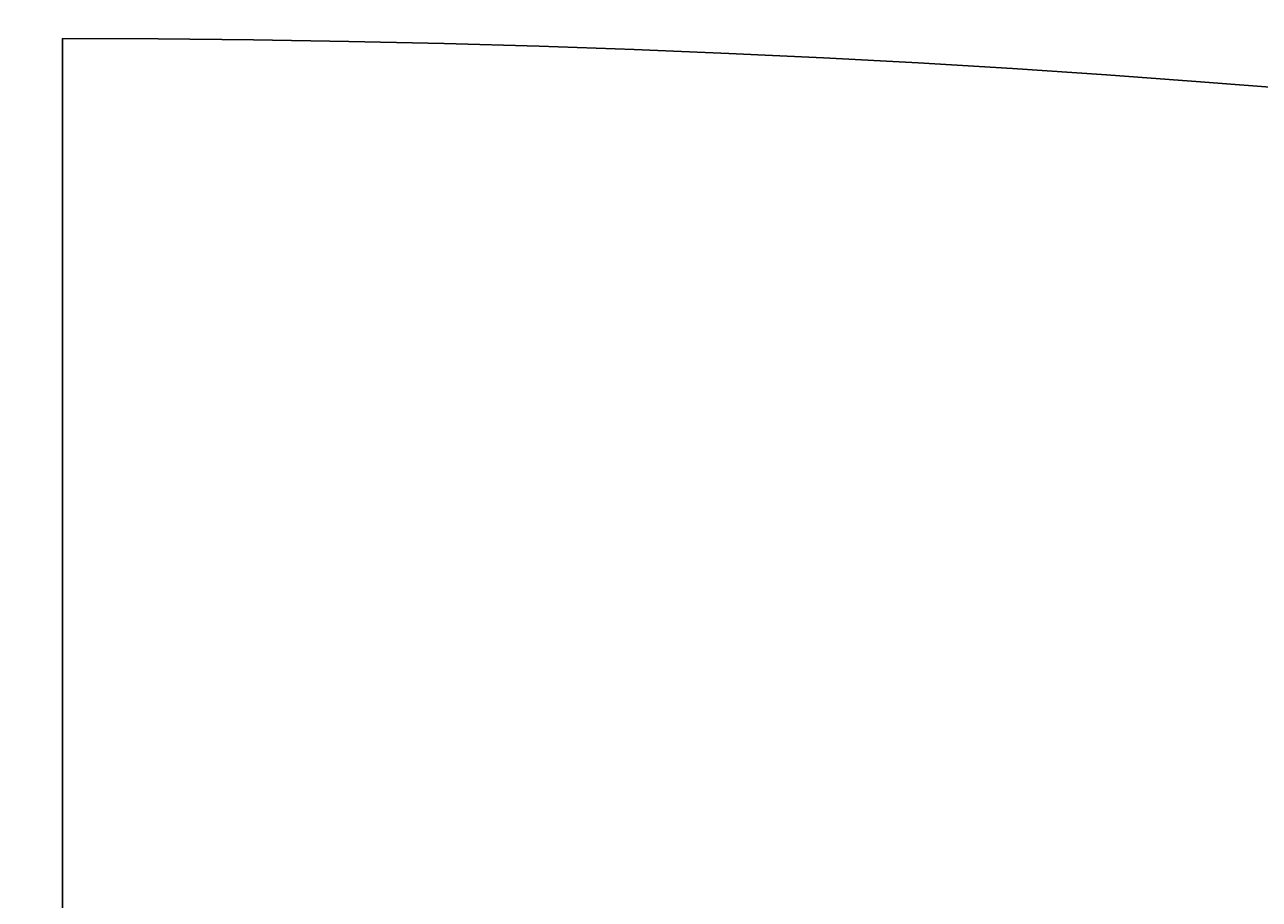
# Model space of a CAD drawing. Units: millimetres. Extents: x 19292 to 100733, y 12374 to 26974.
# Tile 8 of 24: x 29467 to 29528, y 15599 to 15642. Entities that reach past the tile are written whole.
import ezdxf

# ---------------------------------------------------------------- set-up
doc = ezdxf.new("R2010")
doc.units = ezdxf.units.MM
doc.layers.add('A-ANNO-DIMS', color=2, linetype='Continuous', lineweight=18)
doc.layers.add('A-DOOR', color=4, linetype='Continuous', lineweight=25)
doc.styles.get("Standard").update_dxf_attribs({"font": 'arial.ttf'})
doc.dimstyles.get("Standard").update_dxf_attribs({"dimtxt": 0.18, "dimasz": 0.18, "dimexe": 0.18, "dimexo": 0.0625, "dimgap": 0.09, "dimtad": 0, "dimtih": 1, "dimtoh": 1, "dimdec": 4, "dimzin": 0, "dimdsep": 46, "dimtxsty": 'Standard', "dimcen": 0.09, "dimadec": 0, "dimazin": 0, "dimtfac": 1, "dimtdec": 4, "dimtofl": 0, "dimtmove": 0, "dimatfit": 3, "dimfxl": 1, "dimtolj": 1, "dimtzin": 0, "dimarcsym": 0})

# ---------------------------------------------------------------- blocks, each defined once
blk = doc.blocks.new('*D79')
at = {"layer": 'A-ANNO-DIMS', "color": 0, "lineweight": -2, "transparency": 16777216}
for p, q in [((22694.132, 22860.662), (22694.132, 12808.813)), ((36144.169, 15985.662), (36144.169, 12808.813)), ((22694.312, 12808.993), (29418.731, 12808.993)), ((36143.989, 12808.993), (29419.571, 12808.993))]:
    blk.add_line(p, q, dxfattribs=at)
at = {"layer": 'A-ANNO-DIMS', "color": 0, "transparency": 16777216}
for points in [[(22694.312, 12809.023), (22694.312, 12808.963), (22694.132, 12808.993)], [(36143.989, 12809.023), (36143.989, 12808.963), (36144.169, 12808.993)]]:
    blk.add_solid(points, dxfattribs=at)
at = {"layer": 'Defpoints', "color": 0, "transparency": 16777216}
for p in [(22694.132, 22860.725), (36144.169, 15985.725), (36144.169, 12808.993)]:
    blk.add_point(p, dxfattribs=at)
at = {"layer": 'A-ANNO-DIMS', "color": 0, "transparency": 16777216, "insert": (29419.151, 12808.993), "char_height": 0.18, "attachment_point": 5}
blk.add_mtext('\\A1;13450', dxfattribs=at)
blk = doc.blocks.new('*D82')
at = {"layer": 'A-ANNO-DIMS', "color": 0, "lineweight": -2, "transparency": 16777216}
for p, q in [((27198.815, 13562.81), (27198.815, 23555.905)), ((31394.799, 13544.055), (31394.799, 23555.905)), ((27198.995, 23555.725), (29296.444, 23555.725)), ((31394.619, 23555.725), (29297.169, 23555.725))]:
    blk.add_line(p, q, dxfattribs=at)
at = {"layer": 'A-ANNO-DIMS', "color": 0, "transparency": 16777216}
for points in [[(27198.995, 23555.755), (27198.995, 23555.695), (27198.815, 23555.725)], [(31394.619, 23555.755), (31394.619, 23555.695), (31394.799, 23555.725)]]:
    blk.add_solid(points, dxfattribs=at)
at = {"layer": 'Defpoints', "color": 0, "transparency": 16777216}
for p in [(31394.799, 23555.725), (27198.815, 13562.748), (31394.799, 13543.993)]:
    blk.add_point(p, dxfattribs=at)
at = {"layer": 'A-ANNO-DIMS', "color": 0, "transparency": 16777216, "insert": (29296.807, 23555.725), "char_height": 0.18, "attachment_point": 5}
blk.add_mtext('\\A1;4196', dxfattribs=at)
blk = doc.blocks.new('*D86')
at = {"layer": 'A-ANNO-DIMS', "color": 0, "lineweight": -2, "transparency": 16777216}
for p, q in [((27198.815, 15132.81), (27198.815, 23555.905)), ((31198.815, 15132.81), (31198.815, 23555.905)), ((27198.995, 23555.725), (29198.453, 23555.725)), ((31198.635, 23555.725), (29199.177, 23555.725))]:
    blk.add_line(p, q, dxfattribs=at)
at = {"layer": 'A-ANNO-DIMS', "color": 0, "transparency": 16777216}
for points in [[(27198.995, 23555.755), (27198.995, 23555.695), (27198.815, 23555.725)], [(31198.635, 23555.755), (31198.635, 23555.695), (31198.815, 23555.725)]]:
    blk.add_solid(points, dxfattribs=at)
at = {"layer": 'Defpoints', "color": 0, "transparency": 16777216}
for p in [(31198.815, 23555.725), (27198.815, 15132.748), (31198.815, 15132.748)]:
    blk.add_point(p, dxfattribs=at)
at = {"layer": 'A-ANNO-DIMS', "color": 0, "transparency": 16777216, "insert": (29198.815, 23555.725), "char_height": 0.18, "attachment_point": 5}
blk.add_mtext('\\A1;4000', dxfattribs=at)

msp = doc.modelspace()

# ---------------------------------------------------------------- linework, layer by layer
at = {"layer": 'A-DOOR'}
msp.add_line((29468.571, 14906.403), (29468.571, 15641.675), dxfattribs=at)
msp.add_arc((29468.571, 14906.403), 735.272, 0, 90, dxfattribs=at)

# ---------------------------------------------------------------- dimensions: what is measured, and where the dimension line sits
at = {"layer": 'A-ANNO-DIMS'}
for base, p1, p2, picture, middle in [((31394.799, 23555.725), (27198.815, 13562.748), (31394.799, 13543.993), '*D82', (29296.807, 23555.725)), ((31198.815, 23555.725), (27198.815, 15132.748), (31198.815, 15132.748), '*D86', (29198.815, 23555.725)), ((36144.169, 12808.993), (22694.132, 22860.725), (36144.169, 15985.725), '*D79', (29419.151, 12808.993))]:
    dim = msp.add_linear_dim(base=base, p1=p1, p2=p2, dimstyle='Standard', override={"dimdec": 0, "dimlfac": 1, "dimrnd": 0, "dimzin": 0, "dimdsep": 46, "dimlunit": 2}, dxfattribs=at)
    dim.commit()
    dim.dimension.update_dxf_attribs({"geometry": picture, "text_midpoint": middle})

doc.saveas('drawing.dxf')
